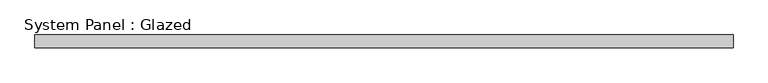
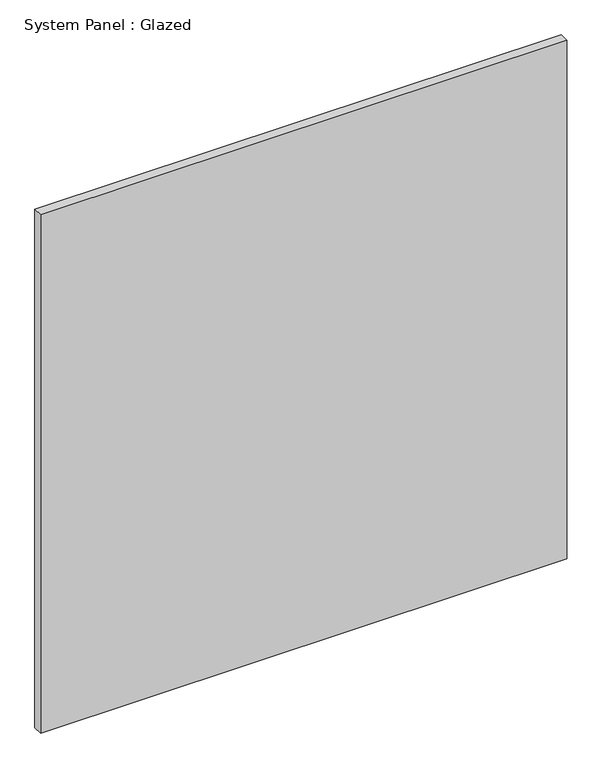
"""IFC4 building model written with IfcOpenShell, lengths in millimetres: plate geometry, System Panel : Glazed."""

from ifc_helpers import new_model, si_unit, origin, origin_with_axes, place, context, project, spatial, polyline, outline, extrude, source, transform, mapped, element, save


def system_panel_glazed_499fa1d4(model_context):
    return source(origin(), model_context, "Body", "SweptSolid", [
        extrude(outline(polyline([(685.8000001, -44.45), (-685.8000001, -44.45), (-685.8000001, -19.05), (685.8000001, -19.05), (685.8000001, -44.45)])), origin_with_axes(), (0.0, 0.0, 1.0), 1428.75),
    ])


if __name__ == "__main__":
    model = new_model("IFC4")
    model_context = context("Model", 3, world=origin())
    ifc_project = project(units=[si_unit("LENGTHUNIT", "METRE", prefix="MILLI")], contexts=[model_context])
    site = spatial("IfcSite", under=ifc_project)
    building = spatial("IfcBuilding", under=site)
    placement = place(None, origin())
    system_panel_glazed_shape = system_panel_glazed_499fa1d4(model_context)
    element("IfcPlate", 1, ObjectType="System Panel : Glazed", at=placement, inside=building, context=model_context, shape_type="MappedRepresentation", body=[
        mapped(system_panel_glazed_shape, transform((0.0, 0.0, 0.0), x_axis=(1.0, 0.0, 0.0), y_axis=(0.0, 1.0, 0.0), z_axis=(0.0, 0.0, 1.0))),
    ])
    save(model, "model.ifc")

# Revit data of these elements
# Type "System Panel : Glazed"
#   Construction Type Id = "GSP4R"
#   Analytic Construction = "1/8 in Pilkington single glazing"
#   Visual Light Transmittance = 0.9
#   Solar Heat Gain Coefficient = 0.86
#   Heat Transfer Coefficient (U) = 1.18115 BTU/(h·ft²·°F)
#   Define Thermal Properties by = 1
# Element 1 (IfcPlate, "System Panel : Glazed")
#   Materials on its faces: "Glass"
# Materials
#   "Glass": class "Glass", colour RGB 0 128 192, transparency 0.75, Description = "Soda Lime Glass", Cost = 0
